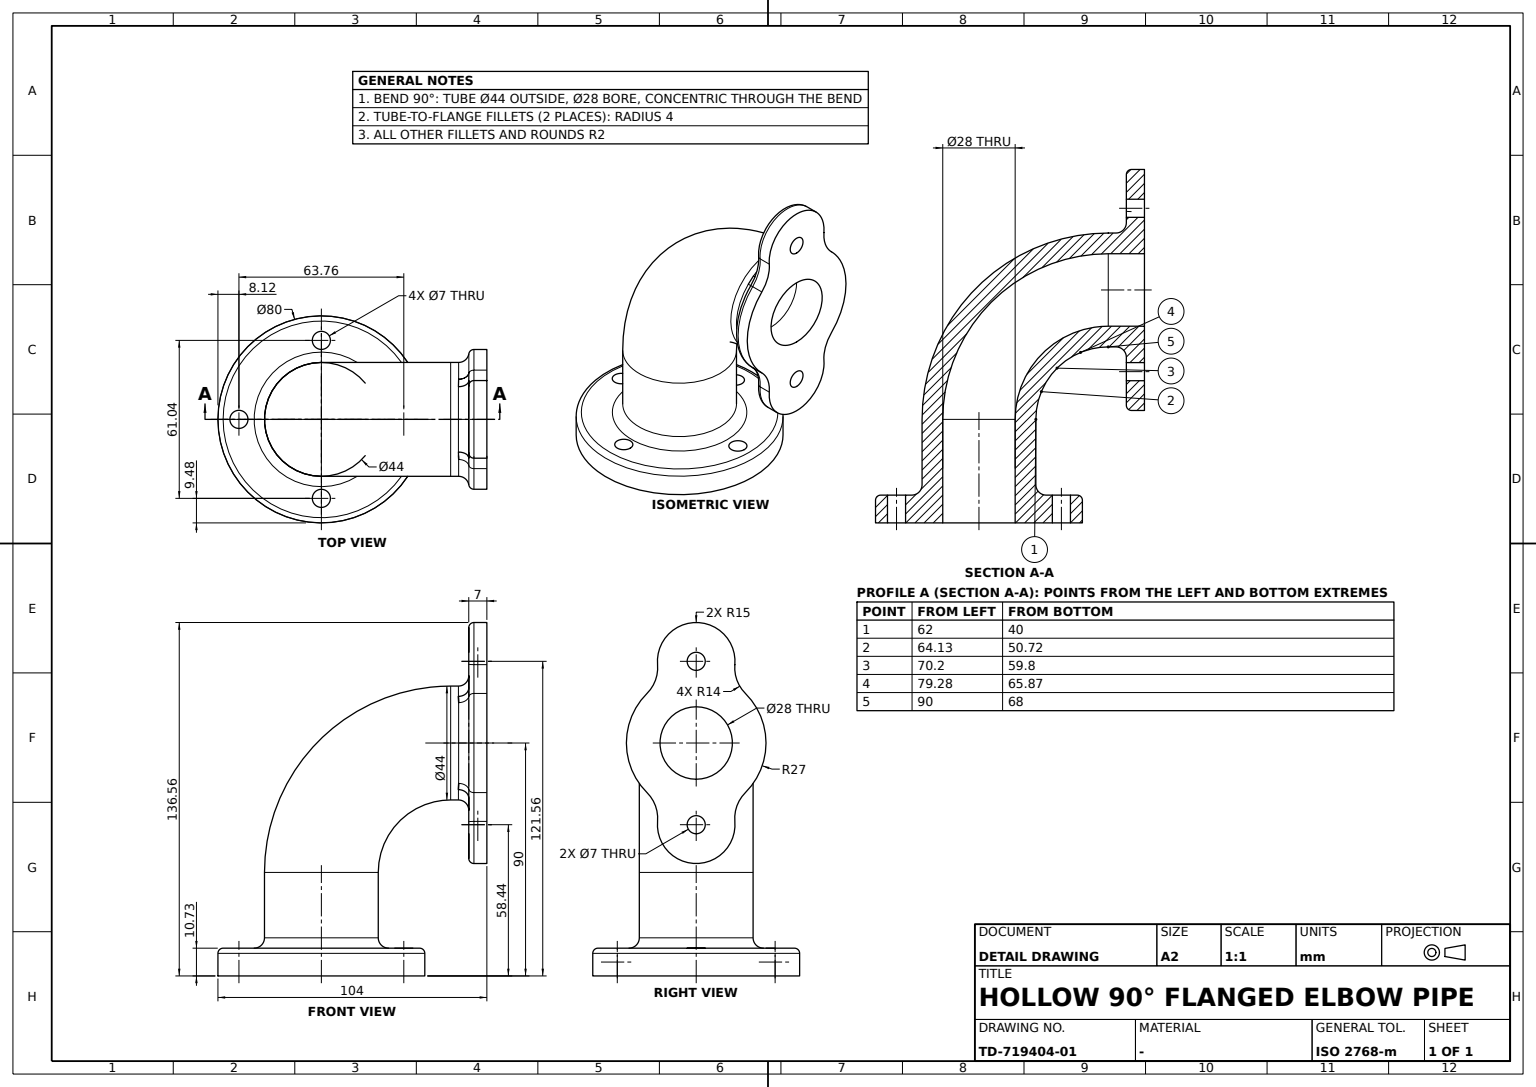
CATIA V5 part; units mm, degrees
sketch "Sketch1" plane through (0, 0, 0) normal (1, 0, 0) x (0, 1, 0)
  line L0 (0, 93.2149) -> (0, -122.7218) construction
  point P0 (0, 93.2149)
  line L1 (-207.0192, 0) -> (181.2672, 0) construction
  point P1 (-207.0192, 0)
  line L2 (14, 40) -> (14, 0)
  point P2 (14, 0)
  line L3 (14, 0) -> (40, 0)
  line L4 (40, 0) -> (40, 8.7298)
  line L5 (38, 10.7298) -> (26, 10.7298)
  point P3 (22, 10.7298)
  line L6 (22, 14.7298) -> (22, 40)
  line L7 (14, 40) -> (22, 40)
  arc A0 (22, 14.7298) -> (26, 10.7298) centre (26, 14.7298) ccw
  arc A1 (38, 10.7298) -> (40, 8.7298) centre (38, 8.7298) cw
  dimension "distance L2 L0" = 14
  dimension "length L2" = 40
  dimension "distance L5 L3" = 10.7298
  dimension "radius A0" = 4
  dimension "distance L6 L0" = 22
  dimension "distance L4 L0" = 40
  dimension "radius A1" = 2
  constraint coincidence P0 y-axis
  constraint coincidence P1 x-axis
  constraint coincidence P2 L1
  constraint coincidence L6 P3
  constraint coincidence L5 P3
  constraint vertical L0 y-axis
  constraint vertical L2 y-axis
  constraint vertical L4 y-axis
  constraint vertical L6 y-axis
  constraint horizontal L1 x-axis
  constraint horizontal L3 x-axis
  constraint horizontal L5 x-axis
  constraint horizontal L7 x-axis
  constraint tangency A0 L6
  constraint tangency A0 L5
  constraint tangency A1 L5
  constraint tangency A1 L4
revolve "Shaft1" add sketch "Sketch1" angle 360 about axis through (0, 0, 0) along (0, 0, 1)
sketch "Sketch2" plane through (0, 0, 40) normal (0, 0, 1) x (1, 0, 0)
  circle A0 centre (0, 0) radius 22
  circle A1 centre (0, 0) radius 14
revolve "Shaft2" add sketch "Sketch2" angle 90 about axis through (50, 0, 40) along (0, 1, 0)
sketch "Sketch3" plane through (0, 0, 10.7298) normal (0, 0, 1) x (1, 0, 0)
  line L0 (0, 45.4908) -> (0, -46.7855) construction
  point P0 (0, 45.4908)
  line L1 (73.9152, 0) -> (-63.2575, 0) construction
  point P1 (73.9152, 0)
  circle A0 centre (0, 30.5188) radius 3.5
  point P2 (0, 30.5188)
  circle A1 centre (-31.8784, 0) radius 3.5
  point P3 (-31.8784, 0)
  circle A2 centre (0, -30.5188) radius 3.5
  point P4 (0, -30.5188)
  point P5 (0, -27.0188)
  circle A3 centre (31.8784, 0) radius 3.5
  point P6 (31.8784, 0)
  dimension "distance P3 P6" = 63.7569
  dimension "distance P2 P4" = 61.0377
  dimension "radius A1" = 3.5
  dimension "radius A0" = 3.5
  dimension "radius A3" = 3.5
  dimension "radius A2" = 3.5
  constraint coincidence P0 y-axis
  constraint coincidence P1 x-axis
  constraint coincidence P2 L0
  constraint coincidence P3 L1
  constraint coincidence P4 L0
  constraint coincidence A2 P5
  constraint coincidence P5 L0
  constraint coincidence P6 L1
  constraint vertical L0 y-axis
  constraint horizontal L1 x-axis
  constraint symmetry P6 P3 L0
  constraint symmetry P4 P2 L1
extrude "Pocket1" cut sketch "Sketch3" against normal up to next
sketch "Sketch4" plane through (50, 0, 0) normal (1, 0, 0) x (0, 1, 0)
  circle A0 centre (0, 90) radius 22
  circle A1 centre (0, 90) radius 14
extrude "Pad1" add sketch "Sketch4" along normal blind 7
sketch "Sketch5" plane through (57, 0, 0) normal (1, 0, 0) x (0, 1, 0)
  circle A0 centre (0, 90) radius 14
  arc A1 (-19.0279, 109.1557) -> (-19.0279, 70.8443) centre (0, 90) ccw
  point P0 (0, 90)
  line L0 (0, 147.6188) -> (0, 16.5629) construction
  point P1 (0, 147.6188)
  line L1 (-90.2015, 90) -> (69.5125, 90) construction
  arc A2 (14.9453, 120.2829) -> (-14.9453, 120.2829) centre (0, 121.5629) ccw
  point P2 (0, 121.5629)
  circle A3 centre (0, 121.5629) radius 3.5
  arc A4 (-19.0279, 109.1557) -> (-14.9453, 120.2829) centre (-28.8942, 119.0882) ccw
  point P3 (-19.0279, 109.1557)
  point P4 (-14.9453, 120.2829)
  arc A5 (14.9453, 120.2829) -> (19.0279, 109.1557) centre (28.8942, 119.0882) ccw
  point P5 (14.9453, 120.2829)
  point P6 (19.0279, 109.1557)
  point P7 (-14.9453, 59.7171)
  point P8 (14.9453, 59.7171)
  arc A6 (14.9453, 59.7171) -> (-14.9453, 59.7171) centre (0, 58.4371) cw
  circle A7 centre (0, 58.4371) radius 3.5
  point P9 (19.0279, 70.8443)
  arc A8 (14.9453, 59.7171) -> (19.0279, 70.8443) centre (28.8942, 60.9118) cw
  point P10 (-19.0279, 70.8443)
  arc A9 (-19.0279, 70.8443) -> (-14.9453, 59.7171) centre (-28.8942, 60.9118) cw
  arc A10 (19.0279, 70.8443) -> (19.0279, 109.1557) centre (0, 90) ccw
  dimension "radius A1" = 27
  dimension "radius A2" = 15
  dimension "radius A3" = 3.5
  dimension "distance A2 L1" = 46.5629
  dimension "radius A4" = 14
  dimension "radius A5" = 14
  constraint concentricity P0 A0
  constraint coincidence P1 y-axis
  constraint coincidence P0 L1
  constraint coincidence P2 L0
  constraint coincidence A1 A10
  constraint vertical L0 y-axis
  constraint horizontal L1 x-axis
  constraint tangency A4 A1
  constraint tangency A4 A2
  constraint tangency A5 A2
  constraint tangency A5 A1
  constraint symmetry P4 P7 L1
  constraint symmetry P5 P8 L1
  constraint symmetry A2 A6 L1
  constraint symmetry A3 A7 L1
  constraint symmetry P6 P9 L1
  constraint symmetry A5 A8 L1
  constraint symmetry P3 P10 L1
  constraint symmetry A4 A9 L1
extrude "Pad2" add sketch "Sketch5" along normal blind 7
fillet "Fillet1" radius 2 1 edges at (57, -27, 90)
fillet "Fillet2" radius 4 1 edges at (57, -22, 90)
sketch "Sketch6" plane through (0, 0, 0) normal (0, 1, 0) x (-1, 0, 0)
